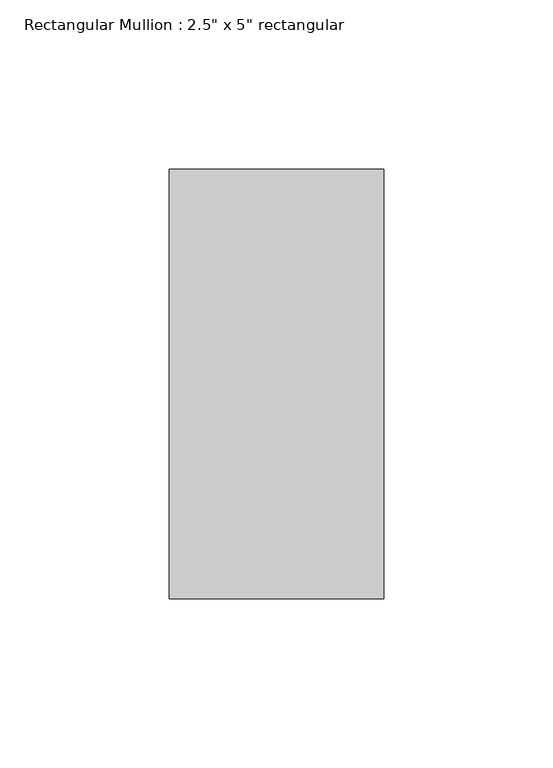
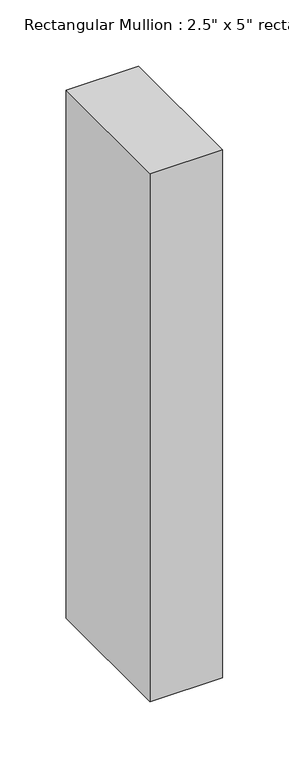
"""IFC4 building model written with IfcOpenShell, lengths in millimetres: member geometry."""

from ifc_helpers import new_model, si_unit, frame, origin, place, context, project, spatial, polyline, outline, extrude, source, transform, mapped, element, save


def member_1750048d(model_context):
    return source(origin(), model_context, "Body", "SweptSolid", [
        extrude(outline(polyline([(31.75, 63.5), (31.75, -63.5), (-31.75, -63.5), (-31.75, 63.5), (31.75, 63.5)])), frame((0.0, 0.0, -487.4598371), z_axis=(0.0, 0.0, 1.0), x_axis=(1.0, 0.0, 0.0)), (0.0, 0.0, 1.0), 487.4598371),
    ])


if __name__ == "__main__":
    model = new_model("IFC4")
    model_context = context("Model", 3, world=origin())
    ifc_project = project(units=[si_unit("LENGTHUNIT", "METRE", prefix="MILLI")], contexts=[model_context])
    site = spatial("IfcSite", under=ifc_project)
    building = spatial("IfcBuilding", under=site)
    placement = place(None, origin())
    member_shape = member_1750048d(model_context)
    element("IfcMember", 1, ObjectType="Rectangular Mullion : 2.5\" x 5\" rectangular", at=placement, inside=building, context=model_context, shape_type="MappedRepresentation", body=[
        mapped(member_shape, transform((0.0, 0.0, 0.0), x_axis=(1.0, 0.0, 0.0), y_axis=(0.0, 1.0, 0.0), z_axis=(0.0, 0.0, 1.0))),
    ])
    save(model, "model.ifc")

# Revit data of these elements
# Type "Rectangular Mullion : 2.5\" x 5\" rectangular"
#   built-in parameter 1007304 = 0.416667 (stored number, unit not read)
#   built-in parameter 1007301 = 0.104167 (stored number, unit not read)
#   built-in parameter 1007300 = 0.104167 (stored number, unit not read)
# Element 1 (IfcMember, "Rectangular Mullion : 2.5\" x 5\" rectangular")
#   Materials on its faces: "mullions"
# Materials
#   "mullions": class "Generic", colour RGB 120 120 120, transparency 0, Cost = 0
